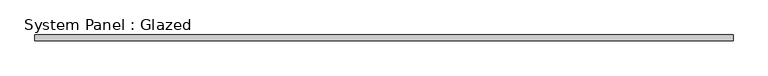
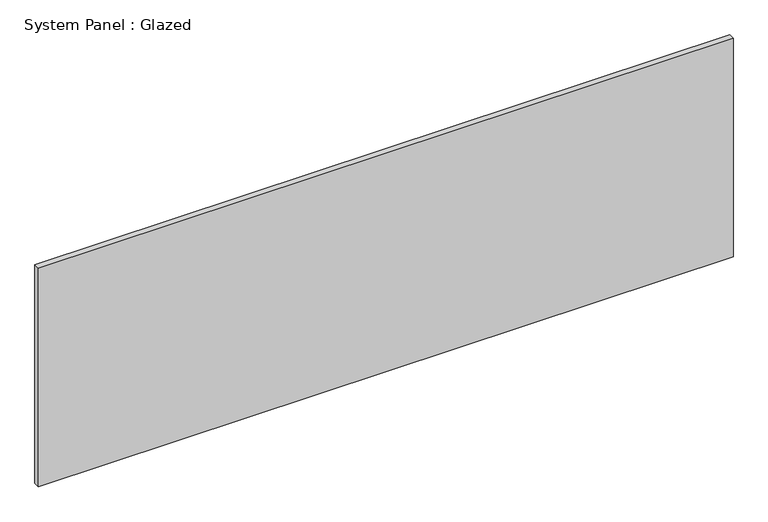
"""IFC4 building model written with IfcOpenShell, lengths in millimetres: plate geometry, System Panel : Glazed."""

from ifc_helpers import new_model, si_unit, origin, origin_with_axes, place, context, project, spatial, polyline, outline, extrude, source, transform, mapped, element, save


def system_panel_glazed_3fab1137(model_context):
    return source(origin(), model_context, "Body", "SweptSolid", [
        extrude(outline(polyline([(1460.5, 19.05), (-1460.5, 19.05), (-1460.5, 44.45), (1460.5, 44.45), (1460.5, 19.05)])), origin_with_axes(), (0.0, 0.0, 1.0), 971.4139568),
    ])


if __name__ == "__main__":
    model = new_model("IFC4")
    model_context = context("Model", 3, world=origin())
    ifc_project = project(units=[si_unit("LENGTHUNIT", "METRE", prefix="MILLI")], contexts=[model_context])
    site = spatial("IfcSite", under=ifc_project)
    building = spatial("IfcBuilding", under=site)
    placement = place(None, origin())
    system_panel_glazed_shape = system_panel_glazed_3fab1137(model_context)
    element("IfcPlate", 1, ObjectType="System Panel : Glazed", at=placement, inside=building, context=model_context, shape_type="MappedRepresentation", body=[
        mapped(system_panel_glazed_shape, transform((0.0, 0.0, 0.0), x_axis=(1.0, 0.0, 0.0), y_axis=(0.0, 1.0, 0.0), z_axis=(0.0, 0.0, 1.0))),
    ])
    save(model, "model.ifc")

# Revit data of these elements
# Type "System Panel : Glazed"
#   Construction Type Id = "GSP4R"
#   Analytic Construction = "1/8 in Pilkington single glazing"
#   Visual Light Transmittance = 0.9
#   Solar Heat Gain Coefficient = 0.86
#   Heat Transfer Coefficient (U) = 1.18115 BTU/(h·ft²·°F)
#   Define Thermal Properties by = 1
# Element 1 (IfcPlate, "System Panel : Glazed")
#   Materials on its faces: "Glass"
# Materials
#   "Glass": class "Glass", colour RGB 0 128 192, transparency 0.75, Description = "Soda Lime Glass", Cost = 0
